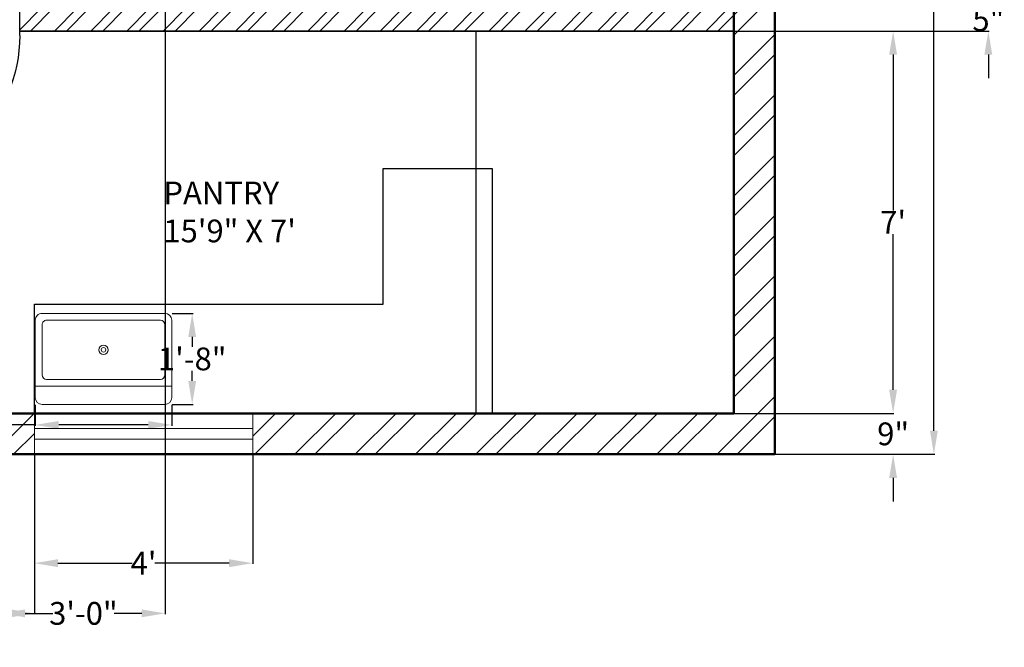
# Model space of a CAD drawing. Units: inches. Extents: x -355 to 263, y -871 to -163.
# Tile 3 of 6: x 23 to 239, y -871 to -733. Entities that reach past the tile are written whole.
import ezdxf

# ---------------------------------------------------------------- set-up
doc = ezdxf.new("R2010")
doc.units = ezdxf.units.IN
doc.header["$MEASUREMENT"] = 0
doc.layers.get('Defpoints').update_dxf_attribs({"color": 50})
for name, color, linetype, lineweight in [('A-ANNO-DIMS', 2, 'Continuous', 18), ('A-AREA-IDEN', 7, 'Continuous', 18), ('A-FLOR-CASE', 9, 'Continuous', 25), ('A-FLOR-FIXT', 8, 'Continuous', 18), ('A-WALL-PATT', 252, 'Continuous', 13)]:
    doc.layers.add(name, color=color, linetype=linetype, lineweight=lineweight)
for name, color, linetype, lineweight, plot in [('DOOR', 4, 'Continuous', 25, False), ('IWAL', 7, 'Continuous', 35, False), ('OWALL', 7, 'Continuous', 50, False), ('WIND', 3, 'Continuous', 18, False)]:
    doc.layers.add(name, color=color, linetype=linetype, lineweight=lineweight, plot=plot)
doc.styles.get("Standard").update_dxf_attribs({"font": 'arial.ttf'})
doc.dimstyles.get("Standard").update_dxf_attribs({"dimtxt": 5, "dimasz": 5.18, "dimexe": 0.18, "dimexo": 0.0625, "dimgap": 0.09, "dimtad": 0, "dimtih": 1, "dimtoh": 1, "dimdec": 0, "dimzin": 0, "dimdsep": 46, "dimlunit": 3, "dimtxsty": 'Standard', "dimcen": 0.09, "dimadec": 0, "dimazin": 0, "dimtfac": 1, "dimtdec": 0, "dimtofl": 0, "dimtmove": 0, "dimatfit": 3, "dimfxl": 1, "dimtolj": 1, "dimtzin": 0, "dimarcsym": 0})

# ---------------------------------------------------------------- blocks, each defined once
blk = doc.blocks.new('*U6')
for p, q in [((0, 0), (0, -6)), ((32, 0), (32, -6))]:
    blk.add_line(p, q)
blk.add_lwpolyline([(0, 0), (0, 32), (1.75, 32), (1.75, 0)], close=True)
blk.add_arc((0, 0), 32, 0, 90)
blk = doc.blocks.new('Sink-single - 30 in top')
blk.add_line((-15, -3.999996), (15, -3.999996))
for points in [[(-13.5, 0), (13.5, 0)], [(-15, -18.499996), (-15, -1.5)], [(15, -1.5), (15, -18.499996)], [(-12.5, -5.499996), (12.5, -5.499996)], [(-13.5, -17.499996), (-13.5, -6.499996)], [(13.5, -6.499996), (13.5, -17.499996)], [(12.5, -18.499996), (-12.5, -18.499996)], [(13.5, -19.999996), (-13.5, -19.999996)]]:
    blk.add_lwpolyline(points)
for radius in [1, 0.5]:
    blk.add_circle((0, -11.999996), radius)
for centre, radius, start, end in [((-13.5, -1.5), 1.5, 90, 180), ((13.5, -1.5), 1.5, 0, 90), ((-12.5, -6.499996), 1, 90, 180), ((12.5, -6.499996), 1, 0, 90), ((-13.5, -18.499996), 1.5, 180, 270), ((-12.5, -17.499996), 1, 180, 270), ((12.5, -17.499996), 1, 270, 0), ((13.5, -18.499996), 1.5, 270, 0)]:
    blk.add_arc(centre, radius, start, end)
blk = doc.blocks.new('*D13')
at = {"layer": 'A-ANNO-DIMS', "color": 0, "lineweight": -2, "transparency": 16777216}
for p, q in [((25.9, -828.34), (25.9, -852.38)), ((73.9, -828.34), (73.9, -852.38)), ((31.08, -852.2), (47.41, -852.2)), ((68.72, -852.2), (52.4, -852.2))]:
    blk.add_line(p, q, dxfattribs=at)
at = {"layer": 'A-ANNO-DIMS', "color": 0, "lineweight": -3, "transparency": 16777216}
for points in [[(31.08, -851.34), (31.08, -853.07), (25.9, -852.2)], [(68.72, -851.34), (68.72, -853.07), (73.9, -852.2)]]:
    blk.add_solid(points, dxfattribs=at)
at = {"layer": 'Defpoints', "color": 0, "lineweight": -3, "transparency": 16777216}
for p in [(25.9, -828.28), (73.9, -828.28), (73.9, -852.2)]:
    blk.add_point(p, dxfattribs=at)
at = {"layer": 'A-ANNO-DIMS', "color": 0, "transparency": 16777216, "insert": (49.9, -852.2), "char_height": 5, "attachment_point": 5}
blk.add_mtext("\\A1;4'", dxfattribs=at)
blk = doc.blocks.new('*D39')
at = {"layer": 'A-ANNO-DIMS', "color": 0, "lineweight": -2, "transparency": 16777216}
for p, q in [((214.67, -814.1), (214.67, -808.92)), ((179.74, -819.28), (214.85, -819.28)), ((188.74, -828.28), (214.85, -828.28)), ((214.67, -833.46), (214.67, -838.64))]:
    blk.add_line(p, q, dxfattribs=at)
at = {"layer": 'A-ANNO-DIMS', "color": 0, "lineweight": -3, "transparency": 16777216}
for points in [[(213.8, -814.1), (215.53, -814.1), (214.67, -819.28)], [(213.8, -833.46), (215.53, -833.46), (214.67, -828.28)]]:
    blk.add_solid(points, dxfattribs=at)
at = {"layer": 'Defpoints', "color": 0, "lineweight": -3, "transparency": 16777216}
for p in [(179.68, -819.28), (214.67, -819.28), (188.68, -828.28)]:
    blk.add_point(p, dxfattribs=at)
at = {"layer": 'A-ANNO-DIMS', "color": 0, "transparency": 16777216, "insert": (214.67, -823.78), "char_height": 5, "attachment_point": 5}
blk.add_mtext('\\A1;9"', dxfattribs=at)
blk = doc.blocks.new('*D40')
at = {"layer": 'A-ANNO-DIMS', "color": 0, "lineweight": -2, "transparency": 16777216}
for p, q in [((179.74, -735.28), (214.85, -735.28)), ((214.67, -740.46), (214.67, -774.69)), ((214.67, -814.1), (214.67, -779.87)), ((179.74, -819.28), (214.85, -819.28))]:
    blk.add_line(p, q, dxfattribs=at)
at = {"layer": 'A-ANNO-DIMS', "color": 0, "lineweight": -3, "transparency": 16777216}
for points in [[(213.8, -740.46), (215.53, -740.46), (214.67, -735.28)], [(213.8, -814.1), (215.53, -814.1), (214.67, -819.28)]]:
    blk.add_solid(points, dxfattribs=at)
at = {"layer": 'Defpoints', "color": 0, "lineweight": -3, "transparency": 16777216}
for p in [(179.68, -735.28), (214.67, -735.28), (179.68, -819.28)]:
    blk.add_point(p, dxfattribs=at)
at = {"layer": 'A-ANNO-DIMS', "color": 0, "transparency": 16777216, "insert": (214.67, -777.28), "char_height": 5, "attachment_point": 5}
blk.add_mtext("\\A1;7'", dxfattribs=at)
blk = doc.blocks.new('*D41')
at = {"layer": 'A-ANNO-DIMS', "color": 0, "lineweight": -2, "transparency": 16777216}
for p, q in [((235.6, -725.1), (235.6, -719.92)), ((188.74, -730.28), (235.78, -730.28)), ((179.74, -735.28), (235.78, -735.28)), ((235.6, -740.46), (235.6, -745.64))]:
    blk.add_line(p, q, dxfattribs=at)
at = {"layer": 'A-ANNO-DIMS', "color": 0, "lineweight": -3, "transparency": 16777216}
for points in [[(234.73, -725.1), (236.46, -725.1), (235.6, -730.28)], [(234.73, -740.46), (236.46, -740.46), (235.6, -735.28)]]:
    blk.add_solid(points, dxfattribs=at)
at = {"layer": 'Defpoints', "color": 0, "lineweight": -3, "transparency": 16777216}
for p in [(188.68, -730.28), (235.6, -730.28), (179.68, -735.28)]:
    blk.add_point(p, dxfattribs=at)
at = {"layer": 'A-ANNO-DIMS', "color": 0, "transparency": 16777216, "insert": (235.6, -732.78), "char_height": 5, "attachment_point": 5}
blk.add_mtext('\\A1;5"', dxfattribs=at)
blk = doc.blocks.new('*D71')
at = {"layer": 'A-ANNO-DIMS', "color": 0, "lineweight": -2, "transparency": 16777216}
for p, q in [((26.1, -817.38), (26.1, -822)), ((56.1, -817.38), (56.1, -822)), ((26.1, -821.82), (20.92, -821.82)), ((50.92, -821.82), (31.28, -821.82))]:
    blk.add_line(p, q, dxfattribs=at)
at = {"layer": 'A-ANNO-DIMS', "color": 0, "lineweight": -3, "transparency": 16777216}
for points in [[(31.28, -820.96), (31.28, -822.68), (26.1, -821.82)], [(50.92, -820.96), (50.92, -822.68), (56.1, -821.82)]]:
    blk.add_solid(points, dxfattribs=at)
at = {"layer": 'Defpoints', "color": 0, "lineweight": -3, "transparency": 16777216}
for p in [(26.1, -817.32), (56.1, -817.32), (26.1, -821.82)]:
    blk.add_point(p, dxfattribs=at)
at = {"layer": 'A-ANNO-DIMS', "color": 0, "transparency": 16777216, "insert": (5.07, -821.82), "char_height": 5, "attachment_point": 5}
blk.add_mtext('\\A1;SINK 2\'-6"', dxfattribs=at)
blk = doc.blocks.new('*D72')
at = {"layer": 'A-ANNO-DIMS', "color": 0, "lineweight": -2, "transparency": 16777216}
for p, q in [((56.16, -797.32), (60.78, -797.32)), ((60.6, -802.5), (60.6, -804.68)), ((60.6, -812.14), (60.6, -809.96)), ((56.16, -817.32), (60.78, -817.32))]:
    blk.add_line(p, q, dxfattribs=at)
at = {"layer": 'A-ANNO-DIMS', "color": 0, "lineweight": -3, "transparency": 16777216}
for points in [[(59.73, -802.5), (61.46, -802.5), (60.6, -797.32)], [(59.73, -812.14), (61.46, -812.14), (60.6, -817.32)]]:
    blk.add_solid(points, dxfattribs=at)
at = {"layer": 'Defpoints', "color": 0, "lineweight": -3, "transparency": 16777216}
for p in [(56.1, -797.32), (56.1, -817.32), (60.6, -817.32)]:
    blk.add_point(p, dxfattribs=at)
at = {"layer": 'A-ANNO-DIMS', "color": 0, "transparency": 16777216, "insert": (60.6, -807.32), "char_height": 5, "attachment_point": 5}
blk.add_mtext('\\A1;1\'-8"', dxfattribs=at)
blk = doc.blocks.new('*D76')
at = {"layer": 'A-ANNO-DIMS', "color": 0, "lineweight": -2, "transparency": 16777216}
for p, q in [((188.74, -216.28), (223.81, -216.28)), ((223.63, -221.46), (223.63, -519.64)), ((223.63, -823.1), (223.63, -524.92)), ((188.74, -828.28), (223.81, -828.28))]:
    blk.add_line(p, q, dxfattribs=at)
at = {"layer": 'A-ANNO-DIMS', "color": 0, "lineweight": -3, "transparency": 16777216}
for points in [[(222.77, -221.46), (224.49, -221.46), (223.63, -216.28)], [(222.77, -823.1), (224.49, -823.1), (223.63, -828.28)]]:
    blk.add_solid(points, dxfattribs=at)
at = {"layer": 'Defpoints', "color": 0, "lineweight": -3, "transparency": 16777216}
for p in [(188.68, -216.28), (223.63, -216.28), (188.68, -828.28)]:
    blk.add_point(p, dxfattribs=at)
at = {"layer": 'A-ANNO-DIMS', "color": 0, "transparency": 16777216, "insert": (223.63, -522.28), "char_height": 5, "attachment_point": 5}
blk.add_mtext('\\A1;51\'-0"', dxfattribs=at)
blk = doc.blocks.new('*D83')
at = {"layer": 'A-ANNO-DIMS', "color": 0, "lineweight": -2, "transparency": 16777216}
for p, q in [((-41.45, -828.34), (-41.45, -863.41)), ((25.9, -828.34), (25.9, -863.41)), ((-36.27, -863.23), (-20.33, -863.23)), ((20.72, -863.23), (4.79, -863.23))]:
    blk.add_line(p, q, dxfattribs=at)
at = {"layer": 'A-ANNO-DIMS', "color": 0, "lineweight": -3, "transparency": 16777216}
for points in [[(-36.27, -862.37), (-36.27, -864.09), (-41.45, -863.23)], [(20.72, -862.37), (20.72, -864.09), (25.9, -863.23)]]:
    blk.add_solid(points, dxfattribs=at)
at = {"layer": 'Defpoints', "color": 0, "lineweight": -3, "transparency": 16777216}
for p in [(-41.45, -828.28), (25.9, -828.28), (25.9, -863.23)]:
    blk.add_point(p, dxfattribs=at)
at = {"layer": 'A-ANNO-DIMS', "color": 0, "transparency": 16777216, "insert": (-7.77, -863.23), "char_height": 5, "attachment_point": 5}
blk.add_mtext('\\A1;5\'-7 1/2"', dxfattribs=at)
blk = doc.blocks.new('*D86')
at = {"layer": 'A-ANNO-DIMS', "color": 0, "lineweight": -2, "transparency": 16777216}
for p, q in [((18.68, -641.34), (18.68, -863.41)), ((54.68, -665.34), (54.68, -863.41)), ((23.86, -863.23), (29.95, -863.23)), ((49.5, -863.23), (43.41, -863.23))]:
    blk.add_line(p, q, dxfattribs=at)
at = {"layer": 'A-ANNO-DIMS', "color": 0, "lineweight": -3, "transparency": 16777216}
for points in [[(23.86, -862.37), (23.86, -864.09), (18.68, -863.23)], [(49.5, -862.37), (49.5, -864.09), (54.68, -863.23)]]:
    blk.add_solid(points, dxfattribs=at)
at = {"layer": 'Defpoints', "color": 0, "lineweight": -3, "transparency": 16777216}
for p in [(18.68, -641.28), (54.68, -665.28), (54.68, -863.23)]:
    blk.add_point(p, dxfattribs=at)
at = {"layer": 'A-ANNO-DIMS', "color": 0, "transparency": 16777216, "insert": (36.68, -863.23), "char_height": 5, "attachment_point": 5}
blk.add_mtext('\\A1;3\'-0"', dxfattribs=at)

msp = doc.modelspace()

# ---------------------------------------------------------------- hatches: boundary and pattern name
at = {"layer": 'A-WALL-PATT'}
h = msp.add_hatch(dxfattribs=at)
h.set_pattern_fill('ANSI32', color=256, scale=25)
h.set_pattern_definition([(45, (-301.32, -828.28), (-6.62913, 6.62913), []), (45, (-296.9, -828.28), (-6.62913, 6.62913), [])])
h.paths.add_polyline_path([(54.68, -289.28), (-301.32, -289.28), (-301.32, -303.28), (-295.02, -303.28), (-292.32, -303.28), (-292.32, -298.28), (54.68, -298.28)])
h.paths.add_polyline_path([(188.68, -216.28), (54.68, -216.28), (54.68, -225.28), (179.68, -225.28), (179.68, -345.28), (179.68, -485.16), (184.18, -485.16), (188.68, -485.16)])
h.paths.add_polyline_path([(188.68, -521.16), (184.18, -521.16), (179.68, -521.16), (179.68, -540.28), (188.68, -540.28)])
h.paths.add_polyline_path([(164.68, -540.28), (155.68, -540.28), (155.68, -552.97), (160.18, -552.97), (164.68, -552.97)])
h.paths.add_polyline_path([(164.68, -588.97), (160.18, -588.97), (155.68, -588.97), (155.68, -620.04), (160.18, -620.04), (164.68, -620.04)])
h.paths.add_polyline_path([(164.68, -656.04), (160.18, -656.04), (155.68, -656.04), (155.68, -682.06), (160.18, -682.06), (164.68, -682.06)])
h.paths.add_polyline_path([(164.68, -718.06), (160.18, -718.06), (155.68, -718.06), (155.68, -730.28), (164.68, -730.28)])
h.paths.add_polyline_path([(188.68, -730.28), (179.68, -730.28), (179.68, -819.28), (73.9, -819.28), (73.9, -823.78), (73.9, -828.28), (188.68, -828.28)])
h.paths.add_polyline_path([(25.9, -819.28), (-41.45, -819.28), (-41.45, -823.78), (-41.45, -828.28), (25.9, -828.28), (25.9, -823.78)])
h.paths.add_polyline_path([(-113.45, -819.28), (-292.32, -819.28), (-292.32, -796.14), (-296.82, -796.14), (-301.32, -796.14), (-301.32, -828.28), (-113.45, -828.28), (-113.45, -823.78)])
h.paths.add_polyline_path([(-292.32, -480.28), (-292.32, -345.28), (-301.32, -345.28), (-301.32, -620.18), (-296.82, -620.18), (-292.32, -620.18)])
h.paths.add_polyline_path([(-292.32, -656.18), (-296.82, -656.18), (-301.32, -656.18), (-301.32, -700.14), (-296.82, -700.14), (-292.32, -700.14)])
h = msp.add_hatch(dxfattribs=at)
h.set_pattern_fill('ANSI32', color=256, scale=15)
h.set_pattern_definition([(45, (-292.3197, -819.28), (-3.977476, 3.977476), []), (45, (-289.668, -819.28), (-3.977476, 3.977476), [])])
h.paths.add_polyline_path([(59.68, -280.18), (57.18, -280.18), (54.68, -280.18), (54.68, -289.28), (54.68, -298.28), (54.68, -303.28), (59.68, -303.28)])
h.paths.add_polyline_path([(59.68, -225.28), (54.68, -225.28), (54.68, -232.18), (57.18, -232.18), (59.68, -232.18)])
h.paths.add_polyline_path([(18.68, -641.28), (18.68, -521.28), (13.68, -521.28), (13.68, -641.28), (-7.32, -665.28), (-105.32, -665.28), (-126.32, -641.28), (-126.32, -521.28), (-131.32, -521.28), (-131.32, -641.28), (-105.32, -670.28), (-7.32, -670.28)])
h.paths.add_polyline_path([(-167.32, -521.28), (-172.32, -521.28), (-172.32, -538.25), (-169.82, -538.25), (-167.32, -538.25)])
h.paths.add_polyline_path([(-134.32, -670.28), (-167.32, -670.28), (-167.32, -610.28), (-167.32, -586.25), (-169.82, -586.25), (-172.32, -586.25), (-172.32, -670.28), (-292.32, -670.28), (-292.32, -675.28), (-139.32, -675.28), (-134.32, -675.28)])
h.paths.add_polyline_path([(-167.32, -345.28), (-172.32, -345.28), (-172.32, -462.28), (-172.32, -480.28), (-292.32, -480.28), (-292.32, -485.28), (-172.32, -485.28), (-167.32, -485.28), (5.68, -485.28), (5.68, -480.28), (-167.32, -480.28)])
h.paths.add_polyline_path([(179.68, -345.28), (30.68, -345.28), (30.68, -365.65), (33.18, -365.65), (35.68, -365.65), (35.68, -350.28), (179.68, -350.28)])
h.paths.add_polyline_path([(-134.32, -707.28), (-139.32, -707.28), (-139.32, -819.28), (-134.32, -819.28)])
h.paths.add_polyline_path([(-9.32, -707.28), (-102.32, -707.28), (-102.32, -712.28), (-14.32, -712.28), (-14.32, -819.28), (-9.32, -819.28)])
h.paths.add_polyline_path([(179.68, -730.28), (22.68, -730.28), (22.68, -735.28), (179.68, -735.28)])
h.paths.add_polyline_path([(179.68, -470.28), (30.68, -470.28), (30.68, -475.28), (54.68, -475.28), (54.68, -505.29), (59.18, -505.29, -0.00418), (59.68, -505.29), (59.68, -475.28), (179.68, -475.28)])
h.paths.add_polyline_path([(35.68, -413.65), (33.18, -413.65), (30.68, -413.65), (30.68, -440.29), (35.18, -440.29, -0.00418), (35.68, -440.29)])
h.paths.add_polyline_path([(179.68, -535.28), (54.68, -535.28), (54.68, -540.28), (54.68, -570.29), (59.18, -570.29, -0.00418), (59.68, -570.29), (59.68, -540.28), (179.68, -540.28)])
h.paths.add_polyline_path([(121.93, -531.51), (160.73, -531.51), (160.73, -512.85), (121.93, -512.85)], flags=9)
h.paths.add_polyline_path([(49.47, -376.48), (111.2, -376.48), (111.2, -357.82), (49.47, -357.82)], flags=9)

# ---------------------------------------------------------------- linework, layer by layer
at = {"layer": 'A-FLOR-CASE'}
for p, q in [((122.95, -735.28), (122.95, -819.28)), ((102.55, -795.28), (102.55, -765.48)), ((102.55, -765.48), (126.55, -765.48)), ((126.55, -765.48), (126.55, -819.28)), ((25.9, -819.28), (25.9, -795.28)), ((25.9, -795.28), (102.55, -795.28))]:
    msp.add_line(p, q, dxfattribs=at)
at = {"layer": 'IWAL'}
msp.add_line((179.68, -735.28), (22.68, -735.28), dxfattribs=at)
at = {"layer": 'OWALL'}
for p, q in [((179.68, -730.28), (179.68, -819.28)), ((188.68, -730.28), (188.68, -828.28)), ((179.68, -819.28), (-292.32, -819.28)), ((188.68, -828.28), (-301.32, -828.28))]:
    msp.add_line(p, q, dxfattribs=at)
at = {"layer": 'WIND'}
for p, q in [((25.9, -823.78), (25.9, -819.28)), ((73.9, -823.78), (73.9, -819.28)), ((25.9, -822.58), (73.9, -822.58)), ((25.9, -823.78), (25.9, -828.28)), ((73.9, -823.78), (73.9, -828.28)), ((25.9, -824.98), (73.9, -824.98))]:
    msp.add_line(p, q, dxfattribs=at)

# ---------------------------------------------------------------- block references
at = {"layer": 'A-FLOR-FIXT', "rotation": 180}
msp.add_blockref('Sink-single - 30 in top', (41.1, -817.32), dxfattribs=at)
at = {"layer": 'DOOR', "xscale": -1, "rotation": 180}
msp.add_blockref('*U6', (-9.32, -736.28), dxfattribs=at)

# ---------------------------------------------------------------- texts
at = {"layer": 'A-AREA-IDEN', "insert": (54.26, -768.36), "char_height": 5, "attachment_point": 1}
msp.add_mtext_dynamic_manual_height_columns('{PANTRY\\P15\'9" X 7\'}', width=56.6621, gutter_width=1, heights=[0], dxfattribs=at)

# ---------------------------------------------------------------- dimensions: what is measured, and where the dimension line sits
at = {"layer": 'A-ANNO-DIMS'}
for base, p1, p2, angle, override, picture, middle in [((223.63, -216.28), (188.68, -828.28), (188.68, -216.28), 90, {"dimdec": 1, "dimlfac": 1, "dimrnd": 0, "dimzin": 1, "dimdsep": 46, "dimlunit": 4, "dimfrac": 2}, '*D76', (223.63, -522.28)), ((214.67, -735.28), (179.68, -819.28), (179.68, -735.28), 270, {"dimclrd": 0, "dimclre": 0, "dimclrt": 0}, '*D40', (214.67, -777.28)), ((60.6, -817.32), (56.1, -797.32), (56.1, -817.32), 270, {"dimdec": 1, "dimlfac": 1, "dimrnd": 0, "dimzin": 1, "dimdsep": 46, "dimlunit": 4, "dimfrac": 2}, '*D72', (60.6, -807.32)), ((214.67, -819.28), (188.68, -828.28), (179.68, -819.28), 270, {"dimclrd": 0, "dimclre": 0, "dimclrt": 0}, '*D39', (214.67, -823.78))]:
    dim = msp.add_linear_dim(base=base, p1=p1, p2=p2, angle=angle, dimstyle='Standard', override=override, dxfattribs=at)
    dim.commit()
    dim.dimension.update_dxf_attribs({"geometry": picture, "text_midpoint": middle})
for base, p1, p2, override, picture, middle in [((54.68, -863.23), (18.68, -641.28), (54.68, -665.28), {"dimdec": 1, "dimlfac": 1, "dimrnd": 0, "dimzin": 1, "dimdsep": 46, "dimlunit": 4, "dimfrac": 2}, '*D86', (36.68, -863.23)), ((25.9042, -863.23), (-41.4512, -828.28), (25.9042, -828.28), {"dimdec": 1, "dimlfac": 1, "dimrnd": 0, "dimzin": 1, "dimdsep": 46, "dimlunit": 4, "dimfrac": 2}, '*D83', (-7.7735, -863.23)), ((73.9, -852.2), (25.9, -828.28), (73.9, -828.28), {"dimclrd": 0, "dimclre": 0, "dimclrt": 0}, '*D13', (49.9, -852.2))]:
    dim = msp.add_linear_dim(base=base, p1=p1, p2=p2, dimstyle='Standard', override=override, dxfattribs=at)
    dim.commit()
    dim.dimension.update_dxf_attribs({"geometry": picture, "text_midpoint": middle})
dim = msp.add_linear_dim(base=(235.6, -730.28), p1=(179.68, -735.28), p2=(188.68, -730.28), angle=270, dimstyle='Standard', override={"dimclrd": 0, "dimclre": 0, "dimclrt": 0}, dxfattribs=at)
dim.commit()
dim.dimension.update_dxf_attribs({"geometry": '*D41', "text_midpoint": (235.6, -732.78), "dimtype": 160})
dim = msp.add_linear_dim(base=(26.1, -821.82), p1=(56.1, -817.32), p2=(26.1, -817.32), angle=180, text='SINK <>', dimstyle='Standard', override={"dimdec": 1, "dimlfac": 1, "dimrnd": 0, "dimzin": 1, "dimdsep": 46, "dimlunit": 4, "dimfrac": 2}, dxfattribs=at)
dim.commit()
dim.dimension.update_dxf_attribs({"geometry": '*D71', "text_midpoint": (5.07, -821.82)})

doc.saveas('drawing.dxf')
